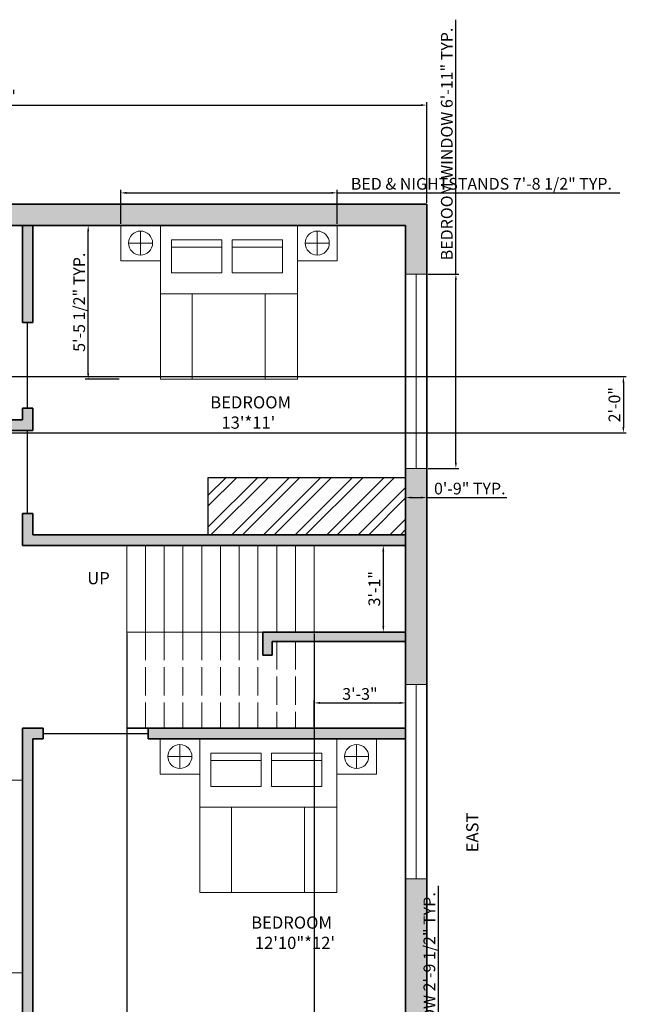
# Model space of a CAD drawing. Units: inches. Extents: x 2066 to 2563, y 1438 to 2142.
# Tile 3 of 3: x 2304 to 2563, y 1710 to 2130. Entities that reach past the tile are written whole.
import ezdxf

# ---------------------------------------------------------------- set-up
doc = ezdxf.new("R2010")
doc.units = ezdxf.units.IN
doc.linetypes.add('ACAD_ISO02W100', pattern=[15, 12, -3])
for name, color, linetype, lineweight in [('A-ANNO-DIMS', 2, 'Continuous', 18), ('A-ANNO-TEXT', 10, 'Continuous', 18), ('A-AREA-IDEN', 10, 'Continuous', 18), ('A-DOOR', 4, 'Continuous', 25), ('A-FLOR-CASE', 191, 'Continuous', 25), ('A-FLOR-CASE-PATT', 9, 'Continuous', 13), ('A-FLOR-STRS', 52, 'Continuous', 18), ('A-FLOR-STRS-OVHD', 52, 'ACAD_ISO02W100', 18), ('A-WALL-PATT', 140, 'Continuous', 13), ('BED', 31, 'Continuous', 18), ('FUR', 191, 'Continuous', 18), ('WALL', 7, 'Continuous', 35), ('WIND', 210, 'Continuous', 18)]:
    doc.layers.add(name, color=color, linetype=linetype, lineweight=lineweight)
doc.styles.get("Standard").update_dxf_attribs({"font": 'arial.ttf'})
doc.dimstyles.new('ISO-25', dxfattribs={"dimtxt": 5, "dimasz": 2.5, "dimexe": 1.25, "dimexo": 0.625, "dimtad": 1, "dimdec": 0, "dimlunit": 4, "dimtxsty": 'Standard', "dimcen": 2.5, "dimadec": 0, "dimazin": 0, "dimtfac": 1, "dimtdec": 0, "dimtmove": 0, "dimatfit": 3, "dimfxl": 1, "dimarcsym": 0})

# ---------------------------------------------------------------- blocks, each defined once
blk = doc.blocks.new('*D6')
at = {"layer": 'A-ANNO-DIMS', "color": 0, "lineweight": -2, "transparency": 16777216}
for p, q in [((2468.45, 1905.54), (2458.29, 1905.54)), ((2459.54, 1903.04), (2459.54, 1871.04)), ((2468.45, 1868.54), (2458.29, 1868.54))]:
    blk.add_line(p, q, dxfattribs=at)
at = {"layer": 'A-ANNO-DIMS', "color": 0, "lineweight": 100, "transparency": 16777216}
for points in [[(2459.12, 1903.04), (2459.96, 1903.04), (2459.54, 1905.54)], [(2459.12, 1871.04), (2459.96, 1871.04), (2459.54, 1868.54)]]:
    blk.add_solid(points, dxfattribs=at)
at = {"layer": 'Defpoints', "color": 0, "lineweight": 100, "transparency": 16777216}
for p in [(2469.07, 1905.54), (2459.54, 1868.54), (2469.07, 1868.54)]:
    blk.add_point(p, dxfattribs=at)
at = {"layer": 'A-ANNO-DIMS', "color": 0, "transparency": 16777216, "insert": (2456.36, 1887.04), "char_height": 5, "attachment_point": 5, "rotation": 90}
blk.add_mtext('3\'-1"', dxfattribs=at)
blk = doc.blocks.new('*D7')
at = {"layer": 'A-ANNO-DIMS', "color": 0, "lineweight": -2, "transparency": 16777216}
for p, q in [((2430.07, 1828.17), (2430.07, 1839.58)), ((2469.07, 1828.17), (2469.07, 1839.58)), ((2432.57, 1838.33), (2466.57, 1838.33))]:
    blk.add_line(p, q, dxfattribs=at)
at = {"layer": 'A-ANNO-DIMS', "color": 0, "lineweight": 100, "transparency": 16777216}
for points in [[(2432.57, 1838.75), (2432.57, 1837.92), (2430.07, 1838.33)], [(2466.57, 1838.75), (2466.57, 1837.92), (2469.07, 1838.33)]]:
    blk.add_solid(points, dxfattribs=at)
at = {"layer": 'Defpoints', "color": 0, "lineweight": 100, "transparency": 16777216}
for p in [(2469.07, 1838.33), (2430.07, 1827.54), (2469.07, 1827.54)]:
    blk.add_point(p, dxfattribs=at)
at = {"layer": 'A-ANNO-DIMS', "color": 0, "transparency": 16777216, "insert": (2449.57, 1841.51), "char_height": 5, "attachment_point": 5}
blk.add_mtext('3\'-3"', dxfattribs=at)
blk = doc.blocks.new('*D8')
at = {"layer": 'A-ANNO-DIMS', "color": 0, "lineweight": -2, "transparency": 16777216}
for p, q in [((2118.07, 2051.67), (2118.07, 2094.59)), ((2120.57, 2093.34), (2475.57, 2093.34)), ((2478.07, 2051.67), (2478.07, 2094.59))]:
    blk.add_line(p, q, dxfattribs=at)
at = {"layer": 'A-ANNO-DIMS', "color": 0, "lineweight": 100, "transparency": 16777216}
for points in [[(2120.57, 2093.76), (2120.57, 2092.93), (2118.07, 2093.34)], [(2475.57, 2093.76), (2475.57, 2092.93), (2478.07, 2093.34)]]:
    blk.add_solid(points, dxfattribs=at)
at = {"layer": 'Defpoints', "color": 0, "lineweight": 100, "transparency": 16777216}
for p in [(2478.07, 2093.34), (2118.07, 2051.04), (2478.07, 2051.04)]:
    blk.add_point(p, dxfattribs=at)
at = {"layer": 'A-ANNO-DIMS', "color": 0, "transparency": 16777216, "insert": (2298.07, 2096.52), "char_height": 5, "attachment_point": 5}
blk.add_mtext("30'", dxfattribs=at)
blk = doc.blocks.new('BED-DOUBLE-WITH-NIGHTSTANDS')
for p, q in [((8.49, 52.9), (8.49, 63.16)), ((83.88, 52.9), (83.88, 63.16)), ((3.36, 58.03), (13.62, 58.03)), ((21.71, 56.35), (43.18, 56.35)), ((47.59, 56.35), (69.05, 56.35)), ((78.75, 58.03), (89.01, 58.03)), ((16.98, 36.37), (75.39, 36.37)), ((30.54, 36.37), (30.54, 0)), ((61.6, 36.37), (61.6, 0))]:
    blk.add_line(p, q)
for points in [[(0, 65.59), (16.98, 65.59), (16.98, 50.47), (0, 50.47)], [(16.98, 65.59), (75.39, 65.59), (75.39, 0), (16.98, 0)], [(75.39, 65.59), (92.37, 65.59), (92.37, 50.47), (75.39, 50.47)], [(21.71, 59.42), (43.18, 59.42), (43.18, 45.29), (21.71, 45.29)], [(47.59, 59.42), (69.05, 59.42), (69.05, 45.29), (47.59, 45.29)]]:
    blk.add_lwpolyline(points, close=True)
for centre in [(8.49, 58.03), (83.88, 58.03)]:
    blk.add_circle(centre, 5.13)
blk = doc.blocks.new('WIN-83IN')
blk.add_line((4.5, 0), (4.5, 82.88))
blk.add_lwpolyline([(0, 82.88), (9, 82.88), (9, 0), (0, 0)], close=True)
blk = doc.blocks.new('*D18')
at = {"layer": 'A-ANNO-DIMS', "color": 0, "lineweight": -2, "transparency": 16777216}
for p, q in [((2347.5, 2042.67), (2347.5, 2057.15)), ((2350, 2055.9), (2437.37, 2055.9)), ((2439.87, 2042.67), (2439.87, 2057.15)), ((2439.87, 2055.9), (2560.43, 2055.9))]:
    blk.add_line(p, q, dxfattribs=at)
at = {"layer": 'A-ANNO-DIMS', "color": 0, "lineweight": 100, "transparency": 16777216}
for points in [[(2350, 2056.31), (2350, 2055.48), (2347.5, 2055.9)], [(2437.37, 2056.31), (2437.37, 2055.48), (2439.87, 2055.9)]]:
    blk.add_solid(points, dxfattribs=at)
at = {"layer": 'Defpoints', "color": 0, "lineweight": 100, "transparency": 16777216}
for p in [(2439.87, 2055.9), (2347.5, 2042.04), (2439.87, 2042.04)]:
    blk.add_point(p, dxfattribs=at)
at = {"layer": 'A-ANNO-DIMS', "color": 0, "transparency": 16777216, "insert": (2501.4, 2059.12), "char_height": 5, "attachment_point": 5}
blk.add_mtext('BED & NIGHTSTANDS 7\'-8 1/2" TYP.', dxfattribs=at)
blk = doc.blocks.new('*D19')
at = {"layer": 'A-ANNO-DIMS', "color": 0, "lineweight": -2, "transparency": 16777216}
for p, q in [((2346.88, 2042.04), (2332.4, 2042.04)), ((2333.65, 1978.95), (2333.65, 2039.54)), ((2346.88, 1976.45), (2332.4, 1976.45))]:
    blk.add_line(p, q, dxfattribs=at)
at = {"layer": 'A-ANNO-DIMS', "color": 0, "lineweight": 100, "transparency": 16777216}
for points in [[(2333.23, 2039.54), (2334.06, 2039.54), (2333.65, 2042.04)], [(2333.23, 1978.95), (2334.06, 1978.95), (2333.65, 1976.45)]]:
    blk.add_solid(points, dxfattribs=at)
at = {"layer": 'Defpoints', "color": 0, "lineweight": 100, "transparency": 16777216}
for p in [(2333.65, 2042.04), (2347.5, 2042.04), (2347.5, 1976.45)]:
    blk.add_point(p, dxfattribs=at)
at = {"layer": 'A-ANNO-DIMS', "color": 0, "transparency": 16777216, "insert": (2330.44, 2009.25), "char_height": 5, "attachment_point": 5, "rotation": 90}
blk.add_mtext('5\'-5 1/2" TYP.', dxfattribs=at)
blk = doc.blocks.new('*D22')
at = {"layer": 'A-ANNO-DIMS', "color": 0, "lineweight": -2, "transparency": 16777216}
for p, q in [((2483.06, 1655.36), (2483.06, 1760.34)), ((2478.7, 1655.36), (2484.31, 1655.36)), ((2483.06, 1624.6), (2483.06, 1652.86)), ((2478.7, 1622.1), (2484.31, 1622.1))]:
    blk.add_line(p, q, dxfattribs=at)
at = {"layer": 'A-ANNO-DIMS', "color": 0, "lineweight": 100, "transparency": 16777216}
for points in [[(2482.64, 1652.86), (2483.48, 1652.86), (2483.06, 1655.36)], [(2482.64, 1624.6), (2483.48, 1624.6), (2483.06, 1622.1)]]:
    blk.add_solid(points, dxfattribs=at)
at = {"layer": 'Defpoints', "color": 0, "lineweight": 100, "transparency": 16777216}
for p in [(2478.07, 1655.36), (2483.06, 1655.36), (2478.07, 1622.1)]:
    blk.add_point(p, dxfattribs=at)
at = {"layer": 'A-ANNO-DIMS', "color": 0, "transparency": 16777216, "insert": (2479.85, 1709.1), "char_height": 5, "attachment_point": 5, "rotation": 90}
blk.add_mtext('TOILET WINDOW 2\'-9 1/2" TYP.', dxfattribs=at)
blk = doc.blocks.new('*D26')
at = {"layer": 'A-ANNO-DIMS', "color": 0, "lineweight": -2, "transparency": 16777216}
for p, q in [((2490.51, 2021.26), (2490.51, 2129.77)), ((2478.7, 2021.26), (2491.76, 2021.26)), ((2490.51, 1940.87), (2490.51, 2018.76)), ((2478.7, 1938.37), (2491.76, 1938.37))]:
    blk.add_line(p, q, dxfattribs=at)
at = {"layer": 'A-ANNO-DIMS', "color": 0, "lineweight": 100, "transparency": 16777216}
for points in [[(2490.09, 2018.76), (2490.92, 2018.76), (2490.51, 2021.26)], [(2490.09, 1940.87), (2490.92, 1940.87), (2490.51, 1938.37)]]:
    blk.add_solid(points, dxfattribs=at)
at = {"layer": 'Defpoints', "color": 0, "lineweight": 100, "transparency": 16777216}
for p in [(2478.07, 2021.26), (2490.51, 2021.26), (2478.07, 1938.37)]:
    blk.add_point(p, dxfattribs=at)
at = {"layer": 'A-ANNO-DIMS', "color": 0, "transparency": 16777216, "insert": (2487.29, 2076.76), "char_height": 5, "attachment_point": 5, "rotation": 90}
blk.add_mtext('BEDROOM WINDOW 6\'-11" TYP.', dxfattribs=at)
blk = doc.blocks.new('*D27')
at = {"layer": 'A-ANNO-DIMS', "color": 0, "lineweight": -2, "transparency": 16777216}
for p, q in [((2469.07, 1937.75), (2469.07, 1924.69)), ((2478.07, 1937.75), (2478.07, 1924.69)), ((2471.57, 1925.94), (2475.57, 1925.94)), ((2478.07, 1925.94), (2512.3, 1925.94))]:
    blk.add_line(p, q, dxfattribs=at)
at = {"layer": 'A-ANNO-DIMS', "color": 0, "lineweight": 100, "transparency": 16777216}
for points in [[(2471.57, 1926.36), (2471.57, 1925.53), (2469.07, 1925.94)], [(2475.57, 1926.36), (2475.57, 1925.53), (2478.07, 1925.94)]]:
    blk.add_solid(points, dxfattribs=at)
at = {"layer": 'Defpoints', "color": 0, "lineweight": 100, "transparency": 16777216}
for p in [(2469.07, 1938.37), (2478.07, 1938.37), (2478.07, 1925.94)]:
    blk.add_point(p, dxfattribs=at)
at = {"layer": 'A-ANNO-DIMS', "color": 0, "transparency": 16777216, "insert": (2496.44, 1929.12), "char_height": 5, "attachment_point": 5}
blk.add_mtext('0\'-9" TYP.', dxfattribs=at)
blk = doc.blocks.new('*D29')
at = {"layer": 'A-ANNO-DIMS', "color": 0, "lineweight": -2, "transparency": 16777216}
for p, q in [((2350.07, 1867.92), (2350.07, 1440.89)), ((2430.07, 1867.92), (2430.07, 1440.89)), ((2352.57, 1442.14), (2427.57, 1442.14))]:
    blk.add_line(p, q, dxfattribs=at)
at = {"layer": 'A-ANNO-DIMS', "color": 0, "lineweight": 100, "transparency": 16777216}
for points in [[(2352.57, 1442.56), (2352.57, 1441.73), (2350.07, 1442.14)], [(2427.57, 1442.56), (2427.57, 1441.73), (2430.07, 1442.14)]]:
    blk.add_solid(points, dxfattribs=at)
at = {"layer": 'Defpoints', "color": 0, "lineweight": 100, "transparency": 16777216}
for p in [(2350.07, 1868.54), (2430.07, 1868.54), (2430.07, 1442.14)]:
    blk.add_point(p, dxfattribs=at)
at = {"layer": 'A-ANNO-DIMS', "color": 0, "transparency": 16777216, "insert": (2390.07, 1445.32), "char_height": 5, "attachment_point": 5}
blk.add_mtext('6\'-8"', dxfattribs=at)
blk = doc.blocks.new('*D33')
at = {"layer": 'A-ANNO-DIMS', "color": 0, "lineweight": -2, "transparency": 16777216}
for p, q in [((2201.63, 1977.54), (2563.22, 1977.54)), ((2561.97, 1975.04), (2561.97, 1956.04)), ((2201.63, 1953.54), (2563.22, 1953.54))]:
    blk.add_line(p, q, dxfattribs=at)
at = {"layer": 'A-ANNO-DIMS', "color": 0, "lineweight": 100, "transparency": 16777216}
for points in [[(2561.56, 1975.04), (2562.39, 1975.04), (2561.97, 1977.54)], [(2561.56, 1956.04), (2562.39, 1956.04), (2561.97, 1953.54)]]:
    blk.add_solid(points, dxfattribs=at)
at = {"layer": 'Defpoints', "color": 0, "lineweight": 100, "transparency": 16777216}
for p in [(2201.01, 1977.54), (2201.01, 1953.54), (2561.97, 1953.54)]:
    blk.add_point(p, dxfattribs=at)
at = {"layer": 'A-ANNO-DIMS', "color": 0, "transparency": 16777216, "insert": (2558.8, 1965.54), "char_height": 5, "attachment_point": 5, "rotation": 90}
blk.add_mtext('2\'-0"', dxfattribs=at)

msp = doc.modelspace()

# ---------------------------------------------------------------- hatches: boundary and pattern name
at = {"layer": 'A-FLOR-CASE-PATT'}
h = msp.add_hatch(dxfattribs=at)
h.set_pattern_fill('ANSI32', color=256)
h.paths.add_polyline_path([(2469.07, 1934.55), (2384.89, 1934.55), (2384.89, 1910.04), (2469.07, 1910.04)])
at = {"layer": 'A-WALL-PATT'}
h = msp.add_hatch(color=256, dxfattribs=at)
h.dxf.hatch_style = 1
h.paths.add_polyline_path([(2210.43, 2051.04), (2194.82, 2051.04), (2194.82, 2042.04), (2210.43, 2042.04)])
h.paths.add_polyline_path([(2265.69, 2051.04), (2243.73, 2051.04), (2243.73, 2042.04), (2265.69, 2042.04)])
h.paths.add_polyline_path([(2478.07, 2051.04), (2288.73, 2051.04), (2288.73, 2042.04), (2288.96, 2042.04), (2469.07, 2042.04), (2469.07, 2021.26), (2478.07, 2021.26)])
h.paths.add_polyline_path([(2127.07, 2042.04), (2134.17, 2042.04), (2134.17, 2051.04), (2118.07, 2051.04), (2118.07, 1957.11), (2127.07, 1957.11), (2127.07, 1977.54)])
h.paths.add_polyline_path([(2201.01, 1982.04), (2127.07, 1982.04), (2127.07, 1977.54), (2201.01, 1977.54)])
h.paths.add_polyline_path([(2247.07, 1982.04), (2241.78, 1982.04), (2241.78, 1977.54), (2247.07, 1977.54)])
h.paths.add_polyline_path([(2251.57, 2042.04), (2247.07, 2042.04), (2247.07, 1954.54), (2310.07, 1954.54), (2310.07, 1964.11), (2305.57, 1964.11), (2305.57, 1959.04), (2251.57, 1959.04)])
h.paths.add_polyline_path([(2310.07, 2042.04), (2305.57, 2042.04), (2305.57, 2000.54), (2310.07, 2000.54)], flags=17)
h.paths.add_polyline_path([(2478.07, 1938.37), (2469.07, 1938.37), (2469.07, 1846.24), (2478.07, 1846.24)])
h.paths.add_polyline_path([(2469.07, 1910.04), (2384.89, 1910.04), (2370.05, 1910.04), (2318.28, 1910.04), (2310.07, 1910.04), (2310.07, 1919.07), (2305.57, 1919.07), (2305.57, 1910.04), (2305.57, 1905.54), (2310.07, 1905.54), (2318.28, 1905.54), (2370.05, 1905.54), (2469.07, 1905.54)])
h.paths.add_polyline_path([(2469.07, 1868.54), (2408.15, 1868.54), (2408.15, 1858.69), (2412.15, 1858.69), (2412.15, 1864.54), (2469.07, 1864.54)])
h.paths.add_polyline_path([(2469.07, 1827.54), (2359.25, 1827.54), (2359.25, 1823.04), (2469.07, 1823.04)])
h.paths.add_polyline_path([(2314.44, 1827.54), (2310.07, 1827.54), (2305.57, 1827.54), (2305.57, 1743.86), (2305.57, 1723.24), (2305.57, 1679.04), (2305.57, 1674.54), (2322.38, 1674.54), (2380.79, 1674.54), (2397.77, 1674.54), (2415.18, 1674.54), (2415.18, 1679.04), (2310.07, 1679.04), (2310.07, 1823.04), (2314.44, 1823.04)])
h.paths.add_polyline_path([(2478.07, 1763.36), (2469.07, 1763.36), (2469.07, 1655.36), (2478.07, 1655.36)])
h.paths.add_polyline_path([(2469.07, 1679.04), (2446.03, 1679.04), (2446.03, 1674.54), (2469.07, 1674.54)])
h.paths.add_polyline_path([(2410.07, 1670.54), (2410.07, 1674.54), (2405.57, 1674.54), (2405.57, 1670.54), (2405.57, 1590.09), (2410.07, 1590.09), (2410.07, 1593.54)])
h.paths.add_polyline_path([(2469.07, 1598.04), (2410.07, 1598.04), (2410.07, 1593.54), (2469.07, 1593.54)])
h.paths.add_polyline_path([(2478.07, 1622.1), (2469.07, 1622.1), (2469.07, 1578.59), (2478.07, 1578.59)])
h.paths.add_polyline_path([(2478.07, 1545.33), (2469.07, 1545.33), (2469.07, 1521.54), (2384.6, 1521.54), (2384.6, 1512.54), (2473.57, 1512.54), (2478.07, 1512.54)])
h.paths.add_polyline_path([(2410.07, 1558.62), (2405.57, 1558.62), (2405.57, 1521.54), (2410.07, 1521.54)])
h.paths.add_polyline_path([(2478.07, 1512.54), (2473.57, 1512.54), (2473.57, 1479.54), (2263.07, 1479.54), (2251.16, 1479.54), (2251.16, 1475.04), (2478.07, 1475.04)])
h.paths.add_polyline_path([(2122.57, 1674.54), (2118.07, 1674.54), (2118.07, 1475.04), (2131.87, 1475.04), (2131.87, 1479.54), (2122.57, 1479.54)])
h.paths.add_polyline_path([(2267.57, 1674.54), (2263.07, 1674.54), (2263.07, 1521.54), (2267.57, 1521.54)])
h.paths.add_polyline_path([(2270.46, 1679.04), (2259.18, 1679.04), (2259.18, 1674.54), (2263.07, 1674.54), (2270.46, 1674.54)])
h.paths.add_polyline_path([(2198.77, 1679.04), (2190.12, 1679.04), (2190.12, 1674.54), (2198.77, 1674.54)])
h.paths.add_polyline_path([(2139.93, 1679.04), (2127.07, 1679.04), (2127.07, 1674.54), (2139.93, 1674.54)])
h.paths.add_polyline_path([(2127.07, 1700.37), (2127.07, 1732.8), (2118.07, 1732.8), (2118.07, 1674.54), (2122.57, 1674.54), (2127.07, 1674.54), (2127.07, 1679.04)])
h.paths.add_polyline_path([(2127.07, 1879.08), (2118.07, 1879.08), (2118.07, 1810.83), (2127.07, 1810.83), (2127.07, 1823.04)])
h.paths.add_polyline_path([(2200.14, 1827.54), (2127.07, 1827.54), (2127.07, 1823.04), (2151.5, 1823.04), (2176.6, 1823.04), (2200.14, 1823.04)])

# ---------------------------------------------------------------- linework, layer by layer
at = {"layer": 'A-DOOR'}
for p, q in [((2307.82, 1964.11), (2307.82, 2000.54)), ((2307.82, 1919.07), (2307.82, 1954.54)), ((2314.44, 1825.29), (2359.25, 1825.29))]:
    msp.add_line(p, q, dxfattribs=at)
at = {"layer": 'A-FLOR-CASE'}
msp.add_lwpolyline([(2469.07, 1910.04), (2384.89, 1910.04), (2384.89, 1934.55), (2469.07, 1934.55)], close=True, dxfattribs=at)
at = {"layer": 'A-FLOR-STRS'}
for p, q in [((2350.07, 1905.54), (2350.07, 1868.54)), ((2358.07, 1905.54), (2358.07, 1868.54)), ((2366.07, 1905.54), (2366.07, 1868.54)), ((2374.07, 1905.54), (2374.07, 1868.54)), ((2382.07, 1905.54), (2382.07, 1868.54)), ((2390.07, 1905.54), (2390.07, 1868.54)), ((2398.07, 1905.54), (2398.07, 1868.54)), ((2406.07, 1905.54), (2406.07, 1868.54)), ((2414.07, 1905.54), (2414.07, 1868.54)), ((2422.07, 1905.54), (2422.07, 1868.54)), ((2430.07, 1905.54), (2430.07, 1868.54)), ((2408.15, 1868.54), (2350.07, 1868.54))]:
    msp.add_line(p, q, dxfattribs=at)
at = {"layer": 'A-FLOR-STRS-OVHD'}
for p, q in [((2350.07, 1868.54), (2350.07, 1827.54)), ((2358.07, 1868.54), (2358.07, 1827.54)), ((2366.07, 1868.54), (2366.07, 1827.54)), ((2374.07, 1868.54), (2374.07, 1827.54)), ((2382.07, 1868.54), (2382.07, 1827.54)), ((2390.07, 1868.54), (2390.07, 1827.54)), ((2398.07, 1868.54), (2398.07, 1827.54)), ((2406.07, 1868.54), (2406.07, 1827.54)), ((2414.07, 1864.54), (2414.07, 1827.54)), ((2422.1, 1864.54), (2422.1, 1827.54)), ((2430.07, 1864.54), (2430.07, 1827.54))]:
    msp.add_line(p, q, dxfattribs=at)
at = {"layer": 'FUR'}
msp.add_lwpolyline([(2305.57, 1805.39), (2297.27, 1805.39), (2297.27, 1723.24), (2305.57, 1723.24)], close=True, dxfattribs=at)
at = {"layer": 'WALL'}
for p, q in [((2118.07, 2051.04), (2478.07, 2051.04)), ((2478.07, 2051.04), (2478.07, 1475.04)), ((2127.07, 2042.04), (2469.07, 2042.04)), ((2305.57, 2042.04), (2305.57, 2000.54)), ((2305.57, 2000.54), (2305.57, 2042.04)), ((2310.07, 2042.04), (2466.07, 2042.04)), ((2310.07, 2042.04), (2310.07, 2000.54)), ((2310.07, 2000.54), (2310.07, 2042.04)), ((2469.07, 2042.04), (2469.07, 1521.54)), ((2305.57, 2000.54), (2310.07, 2000.54)), ((2305.57, 1959.04), (2305.57, 1964.11)), ((2305.57, 1964.11), (2310.07, 1964.11)), ((2305.57, 1964.11), (2305.57, 1959.04)), ((2310.07, 1954.54), (2310.07, 1964.11)), ((2310.07, 1964.11), (2310.07, 1954.54)), ((2251.57, 1959.04), (2305.57, 1959.04)), ((2247.07, 1954.54), (2310.07, 1954.54)), ((2305.57, 1910.04), (2305.57, 1919.07)), ((2310.07, 1919.07), (2305.57, 1919.07)), ((2310.07, 1910.04), (2310.07, 1919.07)), ((2305.57, 1910.04), (2305.57, 1905.54)), ((2310.07, 1910.04), (2318.28, 1910.04)), ((2318.28, 1910.04), (2370.05, 1910.04)), ((2370.05, 1910.04), (2469.07, 1910.04)), ((2310.07, 1905.54), (2305.57, 1905.54)), ((2318.28, 1905.54), (2310.07, 1905.54)), ((2318.28, 1905.54), (2370.05, 1905.54)), ((2370.05, 1905.54), (2469.07, 1905.54)), ((2469.07, 1905.54), (2430.07, 1905.54)), ((2469.07, 1905.54), (2469.07, 1827.54)), ((2469.07, 1905.54), (2469.07, 1866.54)), ((2469.07, 1905.54), (2469.07, 1866.54)), ((2469.07, 1868.54), (2408.15, 1868.54)), ((2408.15, 1858.69), (2408.15, 1868.54)), ((2469.07, 1827.54), (2469.07, 1866.54)), ((2469.07, 1864.54), (2412.15, 1864.54)), ((2412.15, 1864.54), (2412.15, 1858.69)), ((2412.15, 1858.69), (2408.15, 1858.69)), ((2310.07, 1827.54), (2305.57, 1827.54)), ((2305.57, 1827.54), (2305.57, 1743.86)), ((2310.07, 1827.54), (2314.44, 1827.54)), ((2314.44, 1823.04), (2314.44, 1827.54)), ((2350.07, 1827.54), (2469.07, 1827.54)), ((2359.25, 1827.54), (2359.25, 1823.04)), ((2310.07, 1823.04), (2310.07, 1679.04)), ((2310.07, 1679.04), (2310.07, 1823.04)), ((2310.07, 1823.04), (2314.44, 1823.04)), ((2359.25, 1823.04), (2469.07, 1823.04)), ((2305.57, 1743.86), (2305.57, 1679.04))]:
    msp.add_line(p, q, dxfattribs=at)

# ---------------------------------------------------------------- block references
at = {"layer": 'BED'}
for p in [(2347.5, 1976.45), (2364.28, 1757.45)]:
    msp.add_blockref('BED-DOUBLE-WITH-NIGHTSTANDS', p, dxfattribs=at)
at = {"layer": 'WIND'}
for p in [(2469.07, 1938.37), (2469.07, 1763.36)]:
    msp.add_blockref('WIN-83IN', p, dxfattribs=at)

# ---------------------------------------------------------------- texts
at = {"layer": 'A-ANNO-TEXT', "insert": (2333.25, 1894.14), "char_height": 5.193, "attachment_point": 1}
msp.add_mtext_dynamic_manual_height_columns('UP', width=129.7814, gutter_width=25.96, heights=[0], dxfattribs=at)
at = {"layer": 'A-ANNO-TEXT', "insert": (2494.93, 1774.62), "char_height": 5.193, "attachment_point": 1, "rotation": 90}
msp.add_mtext_dynamic_manual_height_columns('EAST', width=129.7814, gutter_width=25.96, heights=[0], dxfattribs=at)
at = {"layer": 'A-AREA-IDEN', "attachment_point": 1}
for s, insert, char_height in [("BEDROOM\\P   13'*11'", (2385.72, 1969.15), 5.193), ('BEDROOM\\P 12\'10"*12\'', (2403.17, 1747.24), 5.1929)]:
    msp.add_mtext_dynamic_manual_height_columns(s, width=129.7814, gutter_width=25.96, heights=[0], dxfattribs=dict(at, insert=insert, char_height=char_height))

# ---------------------------------------------------------------- dimensions: what is measured, and where the dimension line sits
at = {"layer": 'A-ANNO-DIMS'}
for base, p1, p2, text, picture, middle in [((2490.51, 2021.26), (2478.07, 1938.37), (2478.07, 2021.26), 'BEDROOM WINDOW <> TYP.', '*D26', (2487.29, 2076.76)), ((2333.65, 2042.04), (2347.5, 1976.45), (2347.5, 2042.04), '<> TYP.', '*D19', (2330.44, 2009.25)), ((2483.06, 1655.36), (2478.07, 1622.1), (2478.07, 1655.36), 'TOILET WINDOW <> TYP.', '*D22', (2479.85, 1709.1))]:
    dim = msp.add_linear_dim(base=base, p1=p1, p2=p2, angle=90, text=text, dimstyle='ISO-25', override={"dimdec": 1, "dimlfac": 1, "dimrnd": 0, "dimzin": 1, "dimdsep": 46, "dimlunit": 4, "dimfrac": 2}, dxfattribs=at)
    dim.commit()
    dim.dimension.update_dxf_attribs({"geometry": picture, "text_midpoint": middle})
for base, p1, p2, override, picture, middle in [((2478.07, 2093.34), (2118.07, 2051.04), (2478.07, 2051.04), {"dimclrd": 0, "dimclre": 0, "dimclrt": 0}, '*D8', (2298.07, 2096.52)), ((2430.07, 1442.14), (2350.07, 1868.54), (2430.07, 1868.54), {"dimdec": 1, "dimlfac": 1, "dimrnd": 0, "dimzin": 1, "dimdsep": 46, "dimlunit": 4, "dimfrac": 2}, '*D29', (2390.07, 1445.32)), ((2469.07, 1838.33), (2430.07, 1827.54), (2469.07, 1827.54), {"dimclrd": 0, "dimclre": 0, "dimclrt": 0}, '*D7', (2449.57, 1841.51))]:
    dim = msp.add_linear_dim(base=base, p1=p1, p2=p2, dimstyle='ISO-25', override=override, dxfattribs=at)
    dim.commit()
    dim.dimension.update_dxf_attribs({"geometry": picture, "text_midpoint": middle})
for base, p1, p2, text, picture, middle in [((2439.87, 2055.9), (2347.5, 2042.04), (2439.87, 2042.04), 'BED & NIGHTSTANDS <> TYP.', '*D18', (2501.4, 2059.12)), ((2478.07, 1925.94), (2469.07, 1938.37), (2478.07, 1938.37), '<> TYP.', '*D27', (2496.44, 1929.12))]:
    dim = msp.add_linear_dim(base=base, p1=p1, p2=p2, text=text, dimstyle='ISO-25', override={"dimdec": 1, "dimlfac": 1, "dimrnd": 0, "dimzin": 1, "dimdsep": 46, "dimlunit": 4, "dimfrac": 2}, dxfattribs=at)
    dim.commit()
    dim.dimension.update_dxf_attribs({"geometry": picture, "text_midpoint": middle})
for base, p1, p2, override, picture, middle in [((2561.97, 1953.54), (2201.01, 1977.54), (2201.01, 1953.54), {"dimdec": 1, "dimlfac": 1, "dimrnd": 0, "dimzin": 1, "dimdsep": 46, "dimlunit": 4, "dimfrac": 2}, '*D33', (2558.8, 1965.54)), ((2459.54, 1868.54), (2469.07, 1905.54), (2469.07, 1868.54), {"dimclrd": 0, "dimclre": 0, "dimclrt": 0}, '*D6', (2456.36, 1887.04))]:
    dim = msp.add_linear_dim(base=base, p1=p1, p2=p2, angle=90, dimstyle='ISO-25', override=override, dxfattribs=at)
    dim.commit()
    dim.dimension.update_dxf_attribs({"geometry": picture, "text_midpoint": middle})

doc.saveas('drawing.dxf')
